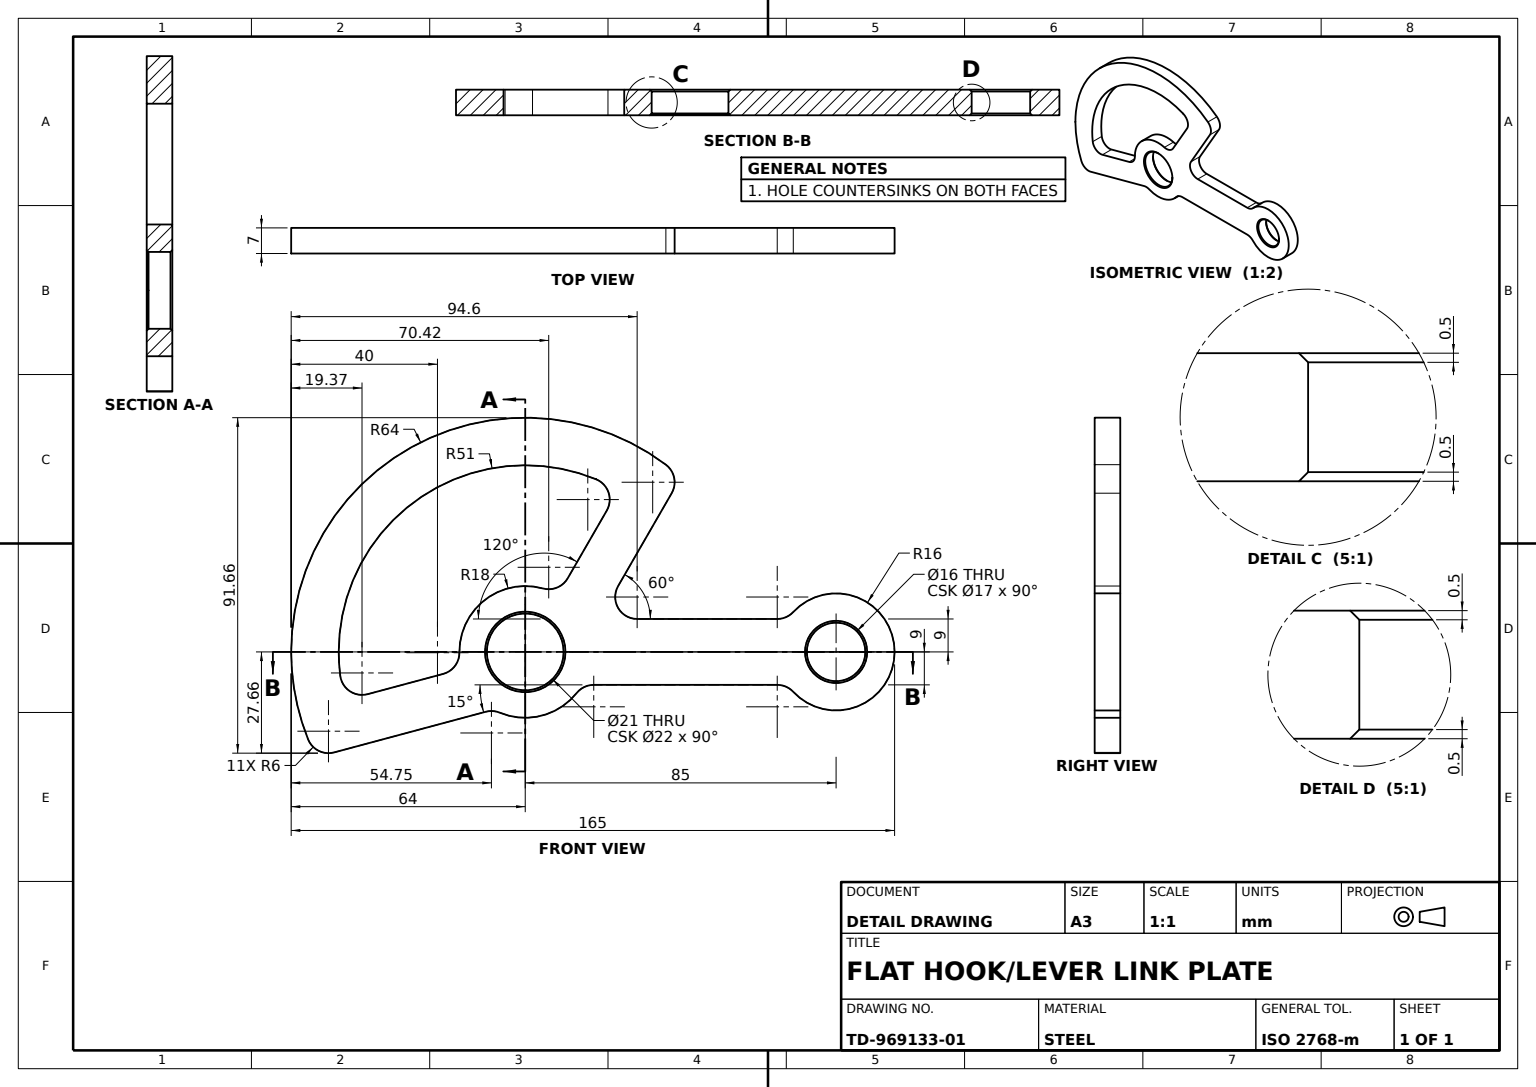
from build123d import *

# Parameters (mm, degrees)
OPENER_PROFILE_SKETCH_R   = 8
OPENER_PROFILE_SKETCH_R_2 = 10.5
OPENER_PLATE_7MM_DEPTH    = 3.5
EDGE_FILLETS_R6_R         = 6
EDGE_CHAMFERS_0_5X45_SIZE = 0.5


with BuildPart() as part:
    # Opener Profile Sketch → Opener Plate 7mm (new, symmetric)
    with BuildSketch(Plane.XY):
        with BuildLine():
            Line((20.207259422, 9), (71.771243445, 9))
            ThreePointArc((71.771243445, 9), (101, 0), (71.771243445, -9))
            Line((71.771243445, -9), (15.588457268, -9))
            ThreePointArc((15.588457268, -9), (4.846344572, -17.335309178), (-8.66103197, -15.779306867))
            Line((-8.66103197, -15.779306867), (-57.165847871, -28.776133117))
            ThreePointArc((-57.165847871, -28.776133117), (-38.960731457, 50.774613779), (42.591220317, 47.770157545))
            Line((42.591220317, 47.770157545), (20.207259422, 9))
        make_face()
        with Locations((85, 0)):
            Circle(OPENER_PROFILE_SKETCH_R, mode=Mode.SUBTRACT)
        Circle(OPENER_PROFILE_SKETCH_R_2, mode=Mode.SUBTRACT)
        with BuildLine():
            Line((9, 15.588457268), (25.5, 44.167295593))
            ThreePointArc((25.5, 44.167295593), (-31.046832879, 40.461020355), (-49.262217141, -13.1997713))
            Line((-49.262217141, -13.1997713), (-17.386664873, -4.658742812))
            ThreePointArc((-17.386664873, -4.658742812), (-10.957705722, 14.280360125), (9, 15.588457268))
        make_face(mode=Mode.SUBTRACT)
    extrude(amount=OPENER_PLATE_7MM_DEPTH, both=True)

    # Edge Fillets R6
    edge_fillets_r6_edges = [part.edges().sort_by_distance(p)[0] for p in [
        (71.771243445, -9, 0),
        (15.588457268, -9, 0),
        (-8.66103197, -15.779306867, 0),
        (-57.165847871, -28.776133117, 0),
        (42.591220317, 47.770157545, 0),
        (20.207259422, 9, 0),
        (71.771243445, 9, 0),
        (-17.386664873, -4.658742812, 0),
        (9, 15.588457268, 0),
        (25.5, 44.167295593, 0),
        (-49.262217141, -13.1997713, 0),
    ]]
    fillet(edge_fillets_r6_edges, radius=EDGE_FILLETS_R6_R)

    # Edge Chamfers 0.5x45
    edge_chamfers_0_5x45_edges = [part.edges().sort_by_distance(p)[0] for p in [
        (77, 0, -3.5),
        (77, 0, 3.5),
        (-10.5, 0, -3.5),
        (-10.5, 0, 3.5),
    ]]
    chamfer(edge_chamfers_0_5x45_edges, length=EDGE_CHAMFERS_0_5X45_SIZE)


solid = part.part
